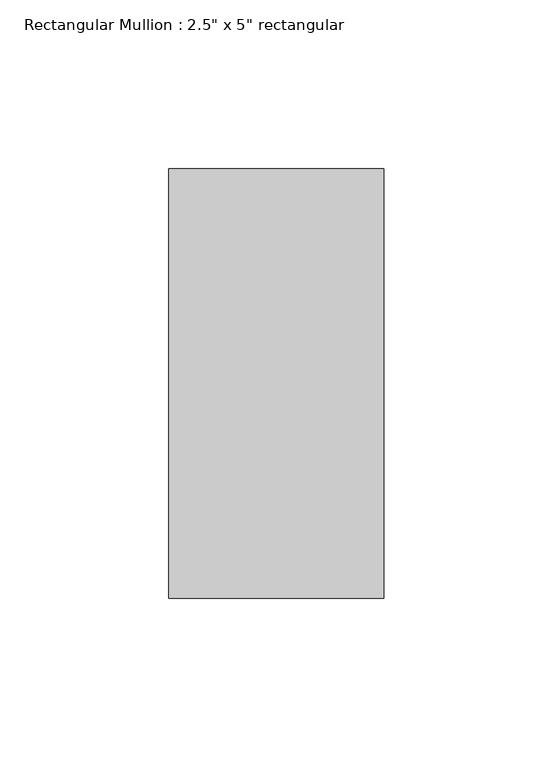
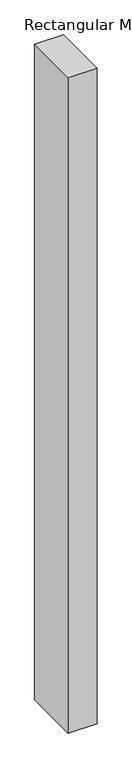
"""IFC4 building model written with IfcOpenShell, lengths in millimetres: member geometry."""

from ifc_helpers import new_model, si_unit, frame, origin, place, context, project, spatial, polyline, outline, extrude, source, transform, mapped, element, save


def member_be902966(model_context):
    return source(origin(), model_context, "Body", "SweptSolid", [
        extrude(outline(polyline([(0.0, 63.5), (0.0, -63.5), (-63.5, -63.5), (-63.5, 63.5), (0.0, 63.5)])), frame((0.0, 0.0, -1522.1457324), z_axis=(0.0, 0.0, 1.0), x_axis=(1.0, 0.0, 0.0)), (0.0, 0.0, 1.0), 1522.1457324),
    ])


if __name__ == "__main__":
    model = new_model("IFC4")
    model_context = context("Model", 3, world=origin())
    ifc_project = project(units=[si_unit("LENGTHUNIT", "METRE", prefix="MILLI")], contexts=[model_context])
    site = spatial("IfcSite", under=ifc_project)
    building = spatial("IfcBuilding", under=site)
    placement = place(None, origin())
    member_shape = member_be902966(model_context)
    element("IfcMember", 1, ObjectType="Rectangular Mullion : 2.5\" x 5\" rectangular", at=placement, inside=building, context=model_context, shape_type="MappedRepresentation", body=[
        mapped(member_shape, transform((0.0, 0.0, 0.0), x_axis=(1.0, 0.0, 0.0), y_axis=(0.0, 1.0, 0.0), z_axis=(0.0, 0.0, 1.0))),
    ])
    save(model, "model.ifc")

# Revit data of these elements
# Type "Rectangular Mullion : 2.5\" x 5\" rectangular"
#   built-in parameter 1007304 = 0.416667 (stored number, unit not read)
#   built-in parameter 1007301 = 0.104167 (stored number, unit not read)
#   built-in parameter 1007300 = 0.104167 (stored number, unit not read)
# Element 1 (IfcMember, "Rectangular Mullion : 2.5\" x 5\" rectangular")
#   Materials on its faces: "Aluminum"
# Materials
#   "Aluminum": class "Metal", colour RGB 247 247 247, transparency 0, Description = "Aluminum 6061", Cost = 0
